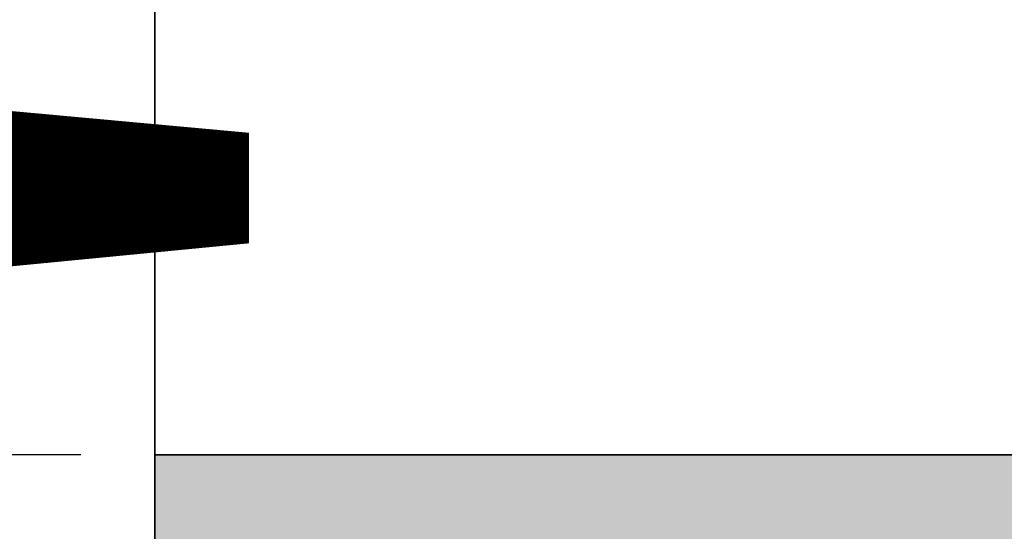
# Model space of a CAD drawing. Units: inches. Extents: x 2083 to 3317, y 1141 to 2115.
# Tile 22 of 256: x 2225.819 to 2234.135, y 1477.116 to 1481.434. Entities that reach past the tile are written whole.
import ezdxf

# ---------------------------------------------------------------- set-up
doc = ezdxf.new("R2010")
doc.units = ezdxf.units.IN
doc.layers.add('A-ANNO-DIMS', color=2, linetype='Continuous', lineweight=18)
doc.layers.add('A-WALL', color=7, linetype='Continuous', lineweight=35)
doc.layers.add('A-WALL-PATT', color=251, linetype='Continuous', lineweight=13, true_color=0x636466)
doc.styles.get("Standard").update_dxf_attribs({"font": 'arial.ttf'})
doc.dimstyles.new('ISO-25', dxfattribs={"dimtxt": 12, "dimasz": 12, "dimexe": 1.25, "dimexo": 0.625, "dimtad": 1, "dimlunit": 3, "dimtxsty": 'Standard', "dimcen": 2.5, "dimadec": 0, "dimazin": 0, "dimtfac": 1, "dimtmove": 0, "dimatfit": 3, "dimfxl": 1, "dimarcsym": 0})

# ---------------------------------------------------------------- blocks, each defined once
blk = doc.blocks.new('*D13')
at = {"layer": 'A-ANNO-DIMS', "color": 0, "lineweight": -2, "transparency": 16777216}
for p, q in [((2226.3348, 1477.7614), (2191.9761, 1477.7614)), ((2193.2261, 1465.7614), (2193.2261, 1275.2614)), ((2226.3348, 1263.2614), (2191.9761, 1263.2614))]:
    blk.add_line(p, q, dxfattribs=at)
at = {"layer": 'A-ANNO-DIMS', "color": 0, "transparency": 16777216}
for points in [[(2191.2261, 1465.7614), (2195.2261, 1465.7614), (2193.2261, 1477.7614)], [(2191.2261, 1275.2614), (2195.2261, 1275.2614), (2193.2261, 1263.2614)]]:
    blk.add_solid(points, dxfattribs=at)
at = {"layer": 'Defpoints', "color": 0, "transparency": 16777216}
for p in [(2226.9598, 1477.7614), (2193.2261, 1263.2614), (2226.9598, 1263.2614)]:
    blk.add_point(p, dxfattribs=at)
at = {"layer": 'A-ANNO-DIMS', "color": 0, "transparency": 16777216, "insert": (2186.4742, 1370.5114), "char_height": 12, "attachment_point": 5, "rotation": 90}
blk.add_mtext('17\'-10.5"', dxfattribs=at)
blk = doc.blocks.new('*D30')
at = {"layer": 'A-ANNO-DIMS', "color": 0, "lineweight": -2, "transparency": 16777216}
for p, q in [((2240.0179, 1445.2738), (2240.0179, 1448.0455)), ((2254.3293, 1445.2738), (2254.3293, 1448.0455)), ((2228.0179, 1446.7955), (2216.0179, 1446.7955)), ((2240.0179, 1446.7955), (2254.3293, 1446.7955)), ((2266.3293, 1446.7955), (2413.7649, 1446.7955))]:
    blk.add_line(p, q, dxfattribs=at)
at = {"layer": 'A-ANNO-DIMS', "color": 0, "transparency": 16777216}
for points in [[(2228.0179, 1448.7955), (2228.0179, 1444.7955), (2240.0179, 1446.7955)], [(2266.3293, 1448.7955), (2266.3293, 1444.7955), (2254.3293, 1446.7955)]]:
    blk.add_solid(points, dxfattribs=at)
at = {"layer": 'Defpoints', "color": 0, "transparency": 16777216}
for p in [(2254.3293, 1446.7955), (2240.0179, 1444.6488), (2254.3293, 1444.6488)]:
    blk.add_point(p, dxfattribs=at)
at = {"layer": 'A-ANNO-DIMS', "color": 0, "transparency": 16777216, "insert": (2346.0471, 1453.6252), "char_height": 12, "attachment_point": 5}
blk.add_mtext('WC 1\'-2 1/2" TYP.', dxfattribs=at)
blk = doc.blocks.new('*D31')
at = {"layer": 'A-ANNO-DIMS', "color": 0, "lineweight": -2, "transparency": 16777216}
for p, q in [((2237.8711, 1456.6488), (2237.8711, 1541.9152)), ((2239.3929, 1444.6488), (2236.6211, 1444.6488)), ((2237.8711, 1431.5475), (2237.8711, 1444.6488)), ((2239.3929, 1431.5475), (2236.6211, 1431.5475)), ((2237.8711, 1419.5475), (2237.8711, 1407.5475))]:
    blk.add_line(p, q, dxfattribs=at)
at = {"layer": 'A-ANNO-DIMS', "color": 0, "transparency": 16777216}
for points in [[(2235.8711, 1456.6488), (2239.8711, 1456.6488), (2237.8711, 1444.6488)], [(2235.8711, 1419.5475), (2239.8711, 1419.5475), (2237.8711, 1431.5475)]]:
    blk.add_solid(points, dxfattribs=at)
at = {"layer": 'Defpoints', "color": 0, "transparency": 16777216}
for p in [(2237.8711, 1444.6488), (2240.0179, 1444.6488), (2240.0179, 1431.5475)]:
    blk.add_point(p, dxfattribs=at)
at = {"layer": 'A-ANNO-DIMS', "color": 0, "transparency": 16777216, "insert": (2231.2175, 1505.282), "char_height": 12, "attachment_point": 5, "rotation": 90}
blk.add_mtext('1\'-1" TYP.', dxfattribs=at)

msp = doc.modelspace()

# ---------------------------------------------------------------- hatches: boundary and pattern name
at = {"layer": 'A-WALL-PATT'}
h = msp.add_hatch(color=256, dxfattribs=at)
h.dxf.hatch_style = 1
h.paths.add_polyline_path([(3126.9598, 2020.7614), (2748.9598, 2020.7614), (2604.9598, 2020.7614), (2226.9598, 2020.7614), (2226.9598, 1702.7614), (2466.9598, 1702.7614), (2466.9598, 1582.7614), (2418.9598, 1582.7614), (2418.9598, 1477.7614), (2226.9598, 1477.7614), (2226.9598, 1263.2614), (2544.9598, 1263.2614), (2544.9598, 1411.7614), (2604.9598, 1411.7614), (2685.9598, 1411.7614), (2685.9598, 1420.7614), (2604.9598, 1420.7614), (2604.9598, 1573.7614), (2604.9598, 1702.7614), (2604.9598, 2011.7614), (2748.9598, 2011.7614), (2748.9598, 1702.7614), (2862.9598, 1702.7614), (2862.9598, 1621.7614), (2871.9598, 1621.7614), (2871.9598, 1702.7614), (2883.9598, 1702.7614), (2883.9598, 1706.9395, -0.026459), (2883.9598, 1711.7614), (2757.9598, 1711.7614), (2757.9598, 1807.7614), (2787.9598, 1807.7614), (2787.9598, 1812.2614), (2757.9598, 1812.2614), (2757.9598, 2011.7614), (2877.9598, 2011.7614), (2877.9598, 1812.2614), (2847.9598, 1812.2614), (2847.9598, 1807.7614), (2889.8357, 1807.7614), (2889.8357, 1812.2614), (2882.4598, 1812.2614), (2882.4598, 2011.7614), (3117.9598, 2011.7614), (3117.9598, 1812.2614), (2937.8357, 1812.2614), (2937.8357, 1807.7614), (2995.7098, 1807.7614), (2995.7098, 1796.1177), (3000.2098, 1796.1177), (3000.2098, 1807.7614), (3117.9598, 1807.7614), (3117.9598, 1711.7614), (3000.2098, 1711.7614), (3000.2098, 1760.1177), (2998.5727, 1760.1177, -0.020711), (2995.7098, 1760.1177), (2995.7098, 1711.7614), (2931.9598, 1711.7614), (2931.9598, 1702.7614), (3126.9598, 1702.7614)])
h.paths.add_polyline_path([(2471.4598, 2011.7614), (2471.4598, 1810.0114), (2462.7169, 1810.0114), (2462.7169, 1805.5114), (2505.9598, 1805.5114), (2505.9598, 1810.0114), (2475.9598, 1810.0114), (2475.9598, 2011.7614), (2595.9598, 2011.7614), (2595.9598, 1810.0114), (2565.9598, 1810.0114), (2565.9598, 1805.5114), (2595.9598, 1805.5114), (2595.9598, 1711.7614), (2235.9598, 1711.7614), (2235.9598, 1805.5114), (2353.7098, 1805.5114), (2353.7098, 1796.0542), (2358.2098, 1796.0542), (2358.2098, 1805.5114), (2414.7169, 1805.5114), (2414.7169, 1810.0114), (2235.9598, 1810.0114), (2235.9598, 2011.7614)], flags=16)
h.paths.add_polyline_path([(2270.2047, 1994.61), (2270.2047, 1970.61), (2246.2047, 1970.61), (2246.2047, 1994.61)], flags=0)
edge = h.paths.add_edge_path(flags=0)
edge.add_ellipse((2332.0274, 1899.7982), major_axis=(-3.043, 3.043), ratio=0.168252, start_angle=-161.33217, end_angle=-156.30711, ccw=False)
edge.add_ellipse((2333.082, 1898.7435), major_axis=(-1.0546, 1.0546), ratio=0.453532, start_angle=-123.37102, end_angle=-94.15911)
edge = h.paths.add_edge_path(flags=0)
edge.add_ellipse((2332.0274, 1968.8763), major_axis=(3.043, 3.043), ratio=0.168252, start_angle=18.66783, end_angle=23.69289)
edge.add_spline(control_points=[(2332.9256, 1970.6911), (2332.2268, 1970.3361), (2330.8937, 1969.6589), (2328.4131, 1970.9321), (2327.2039, 1967.7487), (2324.7096, 1969.9556), (2322.5328, 1967.0124), (2320.0128, 1971.2958), (2317.6803, 1968.1578), (2316.0405, 1967.102), (2315.4269, 1966.8096)], knot_values=[0, 0, 0, 0, 2.267059, 4.324559, 6.685584, 8.878641, 11.121502, 14.300359, 17.755284, 19.732645, 19.732645, 19.732645, 19.732645], degree=3, periodic=0)
edge.add_ellipse((2332.0274, 1968.8763), major_axis=(3.043, 3.043), ratio=0.168252, start_angle=18.66783, end_angle=23.69289, ccw=False)
edge.add_ellipse((2333.082, 1969.9309), major_axis=(1.0546, 1.0546), ratio=0.453532, start_angle=56.62898, end_angle=85.84089, ccw=False)
edge = h.paths.add_edge_path(flags=0)
edge.add_spline(control_points=[(2296.4283, 1967.9879), (2293.6278, 1965.3363), (2287.7036, 1959.7271), (2299.7439, 1949.9957), (2294.5326, 1935.6685), (2290.5732, 1920.6035), (2293.3941, 1909.9737), (2296.1854, 1904.9665)], knot_values=[0.099185, 0.099185, 0.099185, 0.099185, 0.345301, 0.619822, 0.982653, 1.386093, 1.810555, 1.810555, 1.810555, 1.810555], degree=3, periodic=0)
edge.add_spline(control_points=[(2296.1854, 1904.9665), (2297.3836, 1902.6193), (2298.001, 1901.9493), (2298.553, 1901.4682)], knot_values=[0.006246, 0.006246, 0.006246, 0.006246, 0.055476, 0.055476, 0.055476, 0.055476], degree=3, periodic=0)
edge.add_spline(control_points=[(2298.553, 1901.4682), (2297.2586, 1900.9232), (2295.2253, 1900.2321), (2293.0602, 1900.6142), (2292.1014, 1900.7884), (2292.0896, 1900.7906)], knot_values=[0.312835, 0.312835, 0.312835, 0.312835, 0.40178, 0.474987, 0.475903, 0.475903, 0.475903, 0.475903], degree=3, periodic=0)
edge.add_arc((2292.7936, 1904.6641), 3.937, 215.4209, 259.69818, ccw=False)
edge.add_spline(control_points=[(2289.5853, 1902.3823), (2289.4767, 1902.5351), (2289.3685, 1902.688), (2289.2609, 1902.8412)], knot_values=[0.102872, 0.102872, 0.102872, 0.102872, 0.116896, 0.116896, 0.116896, 0.116896], degree=3, periodic=0)
edge.add_spline(control_points=[(2289.2609, 1902.8412), (2288.6866, 1902.5502), (2287.64, 1902.0199), (2285.8813, 1901.874), (2283.853, 1901.5044), (2281.72, 1899.7105), (2278.467, 1899.4929), (2276.1571, 1901.8832), (2272.259, 1899.8041), (2267.7776, 1901.8432), (2262.2439, 1900.184), (2257.4149, 1901.7821), (2254.3184, 1900.7261), (2253.1783, 1900.3373)], knot_values=[0, 0, 0, 0, 1.907977, 3.477176, 5.261074, 7.972851, 11.680248, 13.717921, 16.939592, 22.789562, 27.502503, 33.595215, 37.145618, 37.145618, 37.145618, 37.145618], degree=3, periodic=0)
edge.add_line((2253.1783, 1900.3373), (2250.2442, 1902.8412))
edge.add_line((2250.2442, 1902.8412), (2250.2442, 1965.8333))
edge.add_line((2250.2442, 1965.8333), (2253.1783, 1968.3371))
edge.add_spline(control_points=[(2253.1783, 1968.3371), (2254.3184, 1967.9483), (2257.4149, 1966.8924), (2262.2439, 1968.4904), (2267.7776, 1966.8313), (2271.5267, 1968.5372), (2273.8759, 1967.8283), (2274.2067, 1967.7276)], knot_values=[0, 0, 0, 0, 0.09018, 0.244935, 0.364644, 0.513233, 0.537855, 0.537855, 0.537855, 0.537855], degree=3, periodic=0)
edge.add_arc((2274.3529, 1963.7933), 3.937, 72.05113, 92.12795, ccw=False)
edge.add_arc((2281.2969, 1985.23), 18.5963, 252.05113, 288.56572)
edge.add_arc((2292.3167, 1956.0289), 12.6461, 71.02679, 113.77822, ccw=False)
edge = h.paths.add_edge_path(flags=0)
edge.add_spline(control_points=[(2274.8994, 1951.8562), (2275.0662, 1951.6166), (2275.2327, 1951.3766), (2275.398, 1951.1359)], knot_values=[1.409916, 1.409916, 1.409916, 1.409916, 1.43159, 1.43159, 1.43159, 1.43159], degree=3, periodic=0)
edge.add_spline(control_points=[(2275.398, 1951.1359), (2275.7921, 1950.5619), (2276.1792, 1949.9838), (2276.5455, 1949.3971)], knot_values=[1.358238, 1.358238, 1.358238, 1.358238, 1.409916, 1.409916, 1.409916, 1.409916], degree=3, periodic=0)
edge.add_line((2276.5455, 1949.3971), (2277.4373, 1947.8622))
edge.add_spline(control_points=[(2277.4373, 1947.8622), (2276.3038, 1945.6731), (2274.6397, 1942.4269), (2274.6316, 1938.0939), (2272.7991, 1930.8515), (2274.3564, 1943.897), (2275.9477, 1947.9234), (2276.5455, 1949.3971)], knot_values=[0.005632, 0.005632, 0.005632, 0.005632, 0.186014, 0.266002, 0.357087, 0.59639, 0.739732, 0.739732, 0.739732, 0.739732], degree=3, periodic=0)
edge.add_spline(control_points=[(2276.5455, 1949.3971), (2276.1792, 1949.9838), (2275.7921, 1950.5619), (2275.398, 1951.1359)], knot_values=[1.358238, 1.358238, 1.358238, 1.358238, 1.409916, 1.409916, 1.409916, 1.409916], degree=3, periodic=0)
edge.add_spline(control_points=[(2275.398, 1951.1359), (2274.9425, 1950.0805), (2274.2078, 1948.0253), (2273.9346, 1944.8515), (2272.4685, 1937.6275), (2273.4662, 1945.6965), (2274.7006, 1951.0595), (2274.8994, 1951.8562)], knot_values=[0.104364, 0.104364, 0.104364, 0.104364, 0.189636, 0.269624, 0.36071, 0.600013, 0.644622, 0.644622, 0.644622, 0.644622], degree=3, periodic=0)
h.paths.add_polyline_path([(2269.1675, 1963.1276, -0.357527), (2268.1706, 1960.9764, -0.092561), (2268.1706, 1939.4363, -0.357527), (2269.1675, 1937.2851, -0.357527), (2267.0163, 1938.282, -0.164785), (2254.6856, 1938.282, -0.357527), (2252.5344, 1937.2851, -0.357527), (2253.5313, 1939.4363, -0.092561), (2253.5313, 1960.9764, -0.357527), (2252.5344, 1963.1276, -0.357527), (2254.6856, 1962.1307, -0.164785), (2267.0163, 1962.1307, -0.357527)], flags=0)
h.paths.add_polyline_path([(2248.8741, 1967.8018), (2248.8741, 1957.0277), (2249.4578, 1957.0277), (2249.4578, 1911.6468), (2248.8741, 1911.6468), (2248.8741, 1900.8727), (2246.5119, 1900.8727, 0.197327), (2244.1497, 1902.4569), (2244.1497, 1966.2176, 0.197327), (2246.5119, 1967.8018)], flags=0)
h.paths.add_polyline_path([(2269.1675, 1931.3893, -0.357527), (2268.1706, 1929.2381, -0.092561), (2268.1706, 1907.6981, -0.357527), (2269.1675, 1905.5469, -0.357527), (2267.0163, 1906.5438, -0.164785), (2254.6856, 1906.5438, -0.357527), (2252.5344, 1905.5469, -0.357527), (2253.5313, 1907.6981, -0.092561), (2253.5313, 1929.2381, -0.357527), (2252.5344, 1931.3893, -0.357527), (2254.6856, 1930.3925, -0.164785), (2267.0163, 1930.3925, -0.357527)], flags=0)
edge = h.paths.add_edge_path(flags=0)
edge.add_spline(control_points=[(2276.1969, 1906.7237), (2276.1681, 1909.0289), (2276.114, 1913.3719), (2270.5984, 1924.925), (2273.9052, 1919.0128), (2275.9217, 1916.2621), (2275.4746, 1912.4021), (2277.2579, 1910.3806), (2276.696, 1908.225), (2276.6462, 1906.813), (2276.6178, 1906.0084)], knot_values=[0, 0, 0, 0, 8.61026, 16.221274, 18.843057, 23.804898, 27.440828, 29.356102, 31.203478, 33.650687, 33.650687, 33.650687, 33.650687], degree=3, periodic=0)
edge.add_spline(control_points=[(2276.6178, 1906.0084), (2276.6233, 1905.6241), (2276.4977, 1904.6287), (2275.4418, 1903.8547), (2274.9373, 1903.0804), (2274.8591, 1902.8412)], knot_values=[0.156488, 0.156488, 0.156488, 0.156488, 0.184398, 0.231376, 0.250598, 0.250598, 0.250598, 0.250598], degree=3, periodic=0)
edge.add_line((2274.8591, 1902.8412), (2276.506, 1902.8412))
edge.add_spline(control_points=[(2276.506, 1902.8412), (2276.7883, 1903.0849), (2277.6651, 1904.1252), (2278.2495, 1904.3407), (2277.6539, 1908.5274), (2278.1557, 1906.2278), (2278.1005, 1905.2859), (2278.8467, 1904.069), (2277.8568, 1903.4149), (2277.8742, 1902.991), (2277.9036, 1902.8412)], knot_values=[0.059574, 0.059574, 0.059574, 0.059574, 0.080753, 0.103741, 0.16972, 0.176036, 0.207137, 0.240474, 0.262341, 0.27366, 0.27366, 0.27366, 0.27366], degree=3, periodic=0)
edge.add_line((2277.9036, 1902.8412), (2280.0298, 1902.8412))
edge.add_spline(control_points=[(2280.0298, 1902.8412), (2279.8882, 1903.0884), (2279.4993, 1903.9816), (2280.1523, 1905.9393), (2278.1036, 1909.6578), (2279.7624, 1907.1853), (2280.3279, 1904.8749), (2280.4851, 1903.4896), (2281.4633, 1903.2494), (2281.7583, 1902.9365), (2281.834, 1902.8412)], knot_values=[0.013856, 0.013856, 0.013856, 0.013856, 0.034874, 0.088867, 0.107879, 0.126738, 0.158714, 0.193757, 0.217487, 0.226722, 0.226722, 0.226722, 0.226722], degree=3, periodic=0)
edge.add_spline(control_points=[(2281.834, 1902.8412), (2281.7875, 1902.8267), (2281.647, 1902.783), (2281.3955, 1902.8595), (2281.0881, 1902.9852), (2280.7207, 1903.0609), (2280.3335, 1903.0257), (2280.1248, 1902.8989), (2280.0298, 1902.8412)], knot_values=[0, 0, 0, 0, 0.14413, 0.435517, 0.749276, 1.153046, 1.548371, 1.878348, 1.878348, 1.878348, 1.878348], degree=3, periodic=0)
edge.add_line((2280.0298, 1902.8412), (2277.9036, 1902.8412))
edge.add_spline(control_points=[(2277.9036, 1902.8412), (2277.8929, 1902.7959), (2277.8654, 1902.6796), (2277.6075, 1902.6875), (2277.2741, 1902.8007), (2276.8379, 1902.6198), (2276.5838, 1902.7893), (2276.506, 1902.8412)], knot_values=[0, 0, 0, 0, 0.127189, 0.326199, 0.628009, 1.24357, 1.515331, 1.515331, 1.515331, 1.515331], degree=3, periodic=0)
edge.add_line((2276.506, 1902.8412), (2274.8591, 1902.8412))
edge.add_spline(control_points=[(2274.8591, 1902.8412), (2274.8144, 1902.8986), (2274.7251, 1903.0134), (2274.4935, 1903.119), (2274.2443, 1902.9605), (2273.9371, 1903.1849), (2273.614, 1902.9831), (2273.4083, 1902.883), (2273.3223, 1902.8412)], knot_values=[0, 0, 0, 0, 0.21843, 0.436957, 0.687977, 0.990379, 1.398396, 1.69185, 1.69185, 1.69185, 1.69185], degree=3, periodic=0)
edge.add_spline(control_points=[(2273.3223, 1902.8412), (2273.6167, 1903.4457), (2274.274, 1904.5383), (2276.0272, 1904.5737), (2276.207, 1906.5836), (2276.1969, 1906.7237)], knot_values=[0.012227, 0.012227, 0.012227, 0.012227, 0.059472, 0.106218, 0.134458, 0.134458, 0.134458, 0.134458], degree=3, periodic=0)
h.paths.add_polyline_path([(2270.7761, 1897.7898), (2270.7761, 1873.7898), (2246.7761, 1873.7898), (2246.7761, 1897.7898)], flags=0)
h.paths.add_polyline_path([(2353.7098, 1760.0051), (2353.7098, 1760.0542), (2358.2098, 1760.0542, -0.033729)], flags=0)
h.paths.add_polyline_path([(2321.8191, 1737.5292), (2341.9953, 1737.5292, -0.414214), (2343.2033, 1736.3212), (2343.2033, 1721.0206, -0.414214), (2341.9953, 1719.8127), (2321.8191, 1719.8127, -0.414214), (2320.6112, 1721.0206), (2320.6112, 1736.3212, -0.414214)], flags=0)
h.paths.add_polyline_path([(2324.235, 1736.3212), (2339.5794, 1736.3212, -0.414214), (2341.9953, 1733.9053), (2341.9953, 1725.4497, -0.414214), (2339.5794, 1723.0338), (2333.6806, 1723.0338), (2333.8453, 1722.0455, -0.870646), (2335.4254, 1721.8259, -0.767327), (2333.9227, 1721.4232), (2331.291, 1721.4232, -0.767327), (2329.7883, 1721.8259, -0.870646), (2331.3684, 1722.0455), (2331.5331, 1723.0338), (2324.235, 1723.0338, -0.414214), (2321.8191, 1725.4497), (2321.8191, 1733.9053, -0.414214)], flags=0)
h.paths.add_polyline_path([(2570.4838, 1928.6154), (2589.6838, 1928.6154), (2590.1688, 1928.6154), (2590.1688, 1904.9934), (2570.4838, 1904.9934)], flags=0)
h.paths.add_polyline_path([(2574.4473, 1927.2638, -1), (2572.8288, 1927.2638, -1)], flags=0)
h.paths.add_polyline_path([(2573.0899, 1926.9409), (2573.925, 1927.776), (2574.1477, 1927.5533), (2573.3126, 1926.7182)], flags=0)
h.paths.add_polyline_path([(2578.7791, 1919.7296, -1), (2571.5917, 1919.7296, -1)], flags=0)
h.paths.add_polyline_path([(2578.3854, 1919.7296, -1), (2571.9854, 1919.7296, -1)], flags=0)
h.paths.add_polyline_path([(2331.5958, 1729.4762, -1), (2333.618, 1729.4762, -1)], flags=0)
h.paths.add_polyline_path([(2578.0342, 1927.2638, -1), (2576.4157, 1927.2638, -1)], flags=0)
h.paths.add_polyline_path([(2576.6889, 1927.5311), (2576.9116, 1927.7538), (2577.7467, 1926.9186), (2577.524, 1926.6959)], flags=0)
h.paths.add_polyline_path([(2578.1391, 1909.8595, -1), (2572.2317, 1909.8595, -1)], flags=0)
h.paths.add_polyline_path([(2577.7454, 1909.8595, -1), (2572.6254, 1909.8595, -1)], flags=0)
h.paths.add_polyline_path([(2583.7977, 1927.2638, -1), (2582.1792, 1927.2638, -1)], flags=0)
h.paths.add_polyline_path([(2582.7186, 1927.7538), (2583.5538, 1926.9186), (2583.3311, 1926.6959), (2582.4959, 1927.5311)], flags=0)
h.paths.add_polyline_path([(2582.4959, 1927.5311), (2582.7186, 1927.7538), (2583.5538, 1926.9186), (2583.3311, 1926.6959)], flags=0)
h.paths.add_polyline_path([(2587.7391, 1920.5296, -1), (2581.8317, 1920.5296, -1)], flags=0)
h.paths.add_polyline_path([(2587.3454, 1920.5296, -1), (2582.2254, 1920.5296, -1)], flags=0)
h.paths.add_polyline_path([(2587.3846, 1927.2638, -1), (2585.7661, 1927.2638, -1)], flags=0)
h.paths.add_polyline_path([(2586.082, 1926.9802), (2586.9172, 1927.8154), (2587.1399, 1927.5927), (2586.3047, 1926.7575)], flags=0)
h.paths.add_polyline_path([(2588.3791, 1910.6595, -1), (2581.1917, 1910.6595, -1)], flags=0)
h.paths.add_polyline_path([(2587.9854, 1910.6595, -1), (2581.5854, 1910.6595, -1)], flags=0)
h.paths.add_polyline_path([(2417.1677, 1729.4779), (2437.3439, 1729.4779, -0.414214), (2438.5519, 1728.2699), (2438.5519, 1712.9693, -0.414214), (2437.3439, 1711.7614), (2417.1677, 1711.7614, -0.414214), (2415.9598, 1712.9693), (2415.9598, 1728.2699, -0.414214)], flags=0)
h.paths.add_polyline_path([(2419.5836, 1728.2699), (2434.928, 1728.2699, -0.414214), (2437.3439, 1725.8541), (2437.3439, 1717.3984, -0.414214), (2434.928, 1714.9825), (2429.0292, 1714.9825), (2429.1939, 1713.9942, -0.870646), (2430.774, 1713.7746, -0.767327), (2429.2713, 1713.372), (2426.6396, 1713.372, -0.767327), (2425.1369, 1713.7746, -0.870646), (2426.717, 1713.9942), (2426.8817, 1714.9825), (2419.5836, 1714.9825, -0.414214), (2417.1677, 1717.3984), (2417.1677, 1725.8541, -0.414214)], flags=0)
h.paths.add_polyline_path([(2419.5836, 1728.2699), (2434.928, 1728.2699, -0.414214), (2437.3439, 1725.8541), (2437.3439, 1717.3984, -0.414214), (2434.928, 1714.9825), (2429.0292, 1714.9825), (2428.3581, 1719.009), (2427.5528, 1719.009), (2426.8817, 1714.9825), (2419.5836, 1714.9825, -0.414214), (2417.1677, 1717.3984), (2417.1677, 1725.8541, -0.414214)], flags=0)
h.paths.add_polyline_path([(2426.9444, 1721.4249, -1), (2428.9666, 1721.4249, -1)], flags=0)
h.paths.add_polyline_path([(2475.9598, 1702.7614), (2595.9598, 1702.7614), (2595.9598, 1582.7614), (2475.9598, 1582.7614)], flags=16)
h.paths.add_polyline_path([(2427.9598, 1573.7614), (2595.9598, 1573.7614), (2595.9598, 1468.7614), (2595.9598, 1420.7614), (2384.4598, 1420.7614), (2384.4598, 1468.7614), (2427.9598, 1468.7614)], flags=16)
h.paths.add_polyline_path([(2379.9598, 1468.7614), (2379.9598, 1420.7614), (2235.9598, 1420.7614), (2235.9598, 1468.7614)], flags=16)
h.paths.add_polyline_path([(2317.816, 1466.6958), (2337.9922, 1466.6958, -0.414214), (2339.2002, 1465.4878), (2339.2002, 1450.1872, -0.414214), (2337.9922, 1448.9792), (2317.816, 1448.9792, -0.414214), (2316.6081, 1450.1872), (2316.6081, 1465.4878, -0.414214)], flags=0)
h.paths.add_polyline_path([(2320.2319, 1465.4878), (2335.5763, 1465.4878, -0.414214), (2337.9922, 1463.0719), (2337.9922, 1454.6163, -0.414214), (2335.5763, 1452.2004), (2329.6775, 1452.2004), (2329.8422, 1451.212, -0.870646), (2331.4223, 1450.9925, -0.767327), (2329.9196, 1450.5898), (2327.2879, 1450.5898, -0.767327), (2325.7852, 1450.9925, -0.870646), (2327.3653, 1451.212), (2327.53, 1452.2004), (2320.2319, 1452.2004, -0.414214), (2317.816, 1454.6163), (2317.816, 1463.0719, -0.414214)], flags=0)
h.paths.add_polyline_path([(2320.2319, 1465.4878), (2335.5763, 1465.4878, -0.414214), (2337.9922, 1463.0719), (2337.9922, 1454.6163, -0.414214), (2335.5763, 1452.2004), (2329.6775, 1452.2004), (2329.0064, 1456.2269), (2328.2011, 1456.2269), (2327.53, 1452.2004), (2320.2319, 1452.2004, -0.414214), (2317.816, 1454.6163), (2317.816, 1463.0719, -0.414214)], flags=0)
h.paths.add_polyline_path([(2327.5926, 1458.6428, -1), (2329.6148, 1458.6428, -1)], flags=0)
h.paths.add_polyline_path([(2244.4117, 1433.3405), (2241.9209, 1433.3405, -0.414214), (2240.0179, 1435.2435), (2240.0179, 1440.9528, -0.414211), (2241.9209, 1442.8559), (2244.4117, 1442.8559, -1.976472)], flags=0)
h.paths.add_polyline_path([(2245.3569, 1434.3975, -0.414214), (2245.3569, 1441.7988, -2.144098)], flags=0)
h.paths.add_polyline_path([(2535.9598, 1416.2614), (2535.9598, 1272.2614), (2235.9598, 1272.2614), (2235.9598, 1416.2614)], flags=16)
h.paths.add_polyline_path([(2260.1196, 1384.2928), (2260.1196, 1362.0386), (2237.8654, 1362.0386), (2237.8654, 1384.2928)], flags=0)
edge = h.paths.add_edge_path(flags=0)
edge.add_line((2318.2518, 1362.0933), (2318.1458, 1362.001))
edge.add_ellipse((2317.4451, 1360.431), major_axis=(2.8216, 2.8216), ratio=0.168252, start_angle=18.66783, end_angle=20.94813, ccw=False)
edge.add_ellipse((2318.423, 1361.409), major_axis=(0.9779, 0.9779), ratio=0.453532, start_angle=56.62898, end_angle=70.2262, ccw=False)
edge = h.paths.add_edge_path(flags=0)
edge.add_line((2319.1074, 1295.5711), (2319.015, 1295.6771))
edge.add_ellipse((2317.4451, 1296.3778), major_axis=(-2.8216, 2.8216), ratio=0.168252, start_angle=-161.33217, end_angle=-159.05187, ccw=False)
edge.add_ellipse((2318.423, 1295.3999), major_axis=(-0.9779, 0.9779), ratio=0.453532, start_angle=-123.37102, end_angle=-109.7738)
edge = h.paths.add_edge_path(flags=0)
edge.add_spline(control_points=[(2284.2103, 1301.1702), (2284.5807, 1300.4447), (2284.8912, 1299.892), (2285.1596, 1299.461)], knot_values=[0.039066, 0.039066, 0.039066, 0.039066, 0.055476, 0.055476, 0.055476, 0.055476], degree=3, periodic=0)
edge.add_line((2285.1596, 1299.461), (2284.2103, 1301.1702))
edge = h.paths.add_edge_path(flags=0)
edge.add_line((2280.4125, 1297.298), (2283.37, 1297.0361))
edge.add_line((2283.37, 1297.0361), (2286.4057, 1297.9263))
edge.add_spline(control_points=[(2286.4057, 1297.9263), (2285.3055, 1297.4631), (2284.3448, 1297.1292), (2283.37, 1297.0361)], knot_values=[0.394369, 0.394369, 0.394369, 0.394369, 0.475903, 0.475903, 0.475903, 0.475903], degree=3, periodic=0)
edge.add_spline(control_points=[(2283.37, 1297.0361), (2283.2814, 1297.0277), (2282.3163, 1296.9573), (2281.3125, 1297.1345), (2280.4234, 1297.296), (2280.4125, 1297.298)], knot_values=[0.312835, 0.312835, 0.312835, 0.312835, 0.320246, 0.393453, 0.394369, 0.394369, 0.394369, 0.394369], degree=3, periodic=0)
edge = h.paths.add_edge_path(flags=0)
edge.add_line((2284.4356, 1359.6073), (2280.4463, 1355.328))
edge.add_line((2280.4463, 1355.328), (2279.58, 1351.0178))
edge.add_line((2279.58, 1351.0178), (2282.413, 1346.5804))
edge.add_spline(control_points=[(2282.413, 1346.5804), (2283.1533, 1345.5892), (2284.2529, 1344.0289), (2284.801, 1342.3872), (2284.9352, 1341.8055)], knot_values=[1.240098, 1.240098, 1.240098, 1.240098, 1.332892, 1.382712, 1.382712, 1.382712, 1.382712], degree=3, periodic=0)
edge.add_spline(control_points=[(2284.9352, 1341.8055), (2285.3191, 1340.1406), (2285.233, 1338.4092), (2284.9099, 1336.6541)], knot_values=[1.097484, 1.097484, 1.097484, 1.097484, 1.240098, 1.240098, 1.240098, 1.240098], degree=3, periodic=0)
edge.add_spline(control_points=[(2284.9099, 1336.6541), (2284.5868, 1334.899), (2284.0267, 1333.1203), (2283.4626, 1331.3606)], knot_values=[0.95487, 0.95487, 0.95487, 0.95487, 1.097484, 1.097484, 1.097484, 1.097484], degree=3, periodic=0)
edge.add_line((2283.4626, 1331.3606), (2281.8904, 1326.1534))
edge.add_line((2281.8904, 1326.1534), (2280.7563, 1321.0561))
edge.add_line((2280.7563, 1321.0561), (2280.2992, 1316.002))
edge.add_line((2280.2992, 1316.002), (2280.7159, 1310.9501))
edge.add_line((2280.7159, 1310.9501), (2282.0281, 1305.9721))
edge.add_line((2282.0281, 1305.9721), (2284.2103, 1301.1702))
edge.add_spline(control_points=[(2284.2103, 1301.1702), (2283.3407, 1302.7302), (2282.6119, 1304.3365), (2282.0281, 1305.9721)], knot_values=[0.099185, 0.099185, 0.099185, 0.099185, 0.241799, 0.241799, 0.241799, 0.241799], degree=3, periodic=0)
edge.add_spline(control_points=[(2282.0281, 1305.9721), (2281.4443, 1307.6078), (2281.0055, 1309.2728), (2280.7159, 1310.9501)], knot_values=[0.241799, 0.241799, 0.241799, 0.241799, 0.384413, 0.384413, 0.384413, 0.384413], degree=3, periodic=0)
edge.add_spline(control_points=[(2280.7159, 1310.9501), (2280.4332, 1312.5876), (2280.2894, 1314.277), (2280.2989, 1315.962), (2280.2992, 1316.002)], knot_values=[0.384413, 0.384413, 0.384413, 0.384413, 0.523647, 0.527028, 0.527028, 0.527028, 0.527028], degree=3, periodic=0)
edge.add_spline(control_points=[(2280.2992, 1316.002), (2280.3123, 1317.687), (2280.4779, 1319.3679), (2280.7563, 1321.0561)], knot_values=[0.527028, 0.527028, 0.527028, 0.527028, 0.669642, 0.669642, 0.669642, 0.669642], degree=3, periodic=0)
edge.add_spline(control_points=[(2280.7563, 1321.0561), (2281.0346, 1322.7443), (2281.4259, 1324.4396), (2281.8904, 1326.1534)], knot_values=[0.669642, 0.669642, 0.669642, 0.669642, 0.812256, 0.812256, 0.812256, 0.812256], degree=3, periodic=0)
edge.add_spline(control_points=[(2281.8904, 1326.1534), (2282.2644, 1327.5333), (2282.7879, 1329.2618), (2283.3528, 1331.0178), (2283.4626, 1331.3606)], knot_values=[0.812256, 0.812256, 0.812256, 0.812256, 0.927087, 0.95487, 0.95487, 0.95487, 0.95487], degree=3, periodic=0)
edge.add_line((2283.4626, 1331.3606), (2284.9099, 1336.6541))
edge.add_line((2284.9099, 1336.6541), (2284.9352, 1341.8055))
edge.add_line((2284.9352, 1341.8055), (2282.413, 1346.5804))
edge.add_spline(control_points=[(2282.413, 1346.5804), (2281.2751, 1348.1038), (2280.0784, 1349.5703), (2279.58, 1351.0178)], knot_values=[1.382712, 1.382712, 1.382712, 1.382712, 1.525326, 1.525326, 1.525326, 1.525326], degree=3, periodic=0)
edge.add_spline(control_points=[(2279.58, 1351.0178), (2279.4433, 1351.4147), (2279.1363, 1352.8569), (2279.7352, 1354.2904), (2280.4463, 1355.328)], knot_values=[1.525326, 1.525326, 1.525326, 1.525326, 1.564439, 1.667941, 1.667941, 1.667941, 1.667941], degree=3, periodic=0)
edge.add_spline(control_points=[(2280.4463, 1355.328), (2281.4261, 1356.7578), (2282.9308, 1358.1826), (2284.4356, 1359.6073)], knot_values=[1.667941, 1.667941, 1.667941, 1.667941, 1.810555, 1.810555, 1.810555, 1.810555], degree=3, periodic=0)
edge.add_arc((2280.6231, 1348.5182), 11.7262, 71.02679, 113.77822)
edge.add_arc((2270.4049, 1375.5952), 17.2436, 252.05113, 288.56572, ccw=False)
edge.add_arc((2263.966, 1355.7178), 3.6506, 72.05113, 92.12795)
edge.add_arc((2263.966, 1355.7178), 3.6506, 92.12795, 177.98513)
edge.add_spline(control_points=[(2260.3176, 1355.8462), (2260.2604, 1354.2207), (2260.5513, 1350.1865), (2262.9993, 1346.7663), (2264.4727, 1344.649)], knot_values=[1.43159, 1.43159, 1.43159, 1.43159, 1.564144, 1.770695, 1.770695, 1.770695, 1.770695], degree=3, periodic=0)
edge.add_line((2264.4727, 1344.649), (2264.9356, 1343.9825))
edge.add_spline(control_points=[(2263.801, 1340.2481), (2263.8432, 1340.5141), (2264.0672, 1341.7565), (2264.5127, 1343.0025), (2264.935, 1343.9811)], knot_values=[0.53657, 0.53657, 0.53657, 0.53657, 0.559349, 0.644622, 0.644622, 0.644622, 0.644622], degree=3, periodic=0)
edge.add_spline(control_points=[(2264.935, 1343.9811), (2265.1178, 1343.715), (2265.2989, 1343.4479), (2265.4768, 1343.1794)], knot_values=[1.384077, 1.384077, 1.384077, 1.384077, 1.409916, 1.409916, 1.409916, 1.409916], degree=3, periodic=0)
edge.add_spline(control_points=[(2265.4768, 1343.1794), (2265.6546, 1342.9108), (2265.8293, 1342.6408), (2265.9991, 1342.3688)], knot_values=[1.358238, 1.358238, 1.358238, 1.358238, 1.384077, 1.384077, 1.384077, 1.384077], degree=3, periodic=0)
edge.add_line((2265.9991, 1342.3688), (2266.826, 1340.9455))
edge.add_spline(control_points=[(2266.826, 1340.9455), (2268.8944, 1337.0897), (2271.3982, 1325.843), (2270.5162, 1310.5686), (2275.9194, 1301.8606), (2277.7895, 1299.1994)], knot_values=[0.116896, 0.116896, 0.116896, 0.116896, 0.472987, 1.050969, 1.313793, 1.313793, 1.313793, 1.313793], degree=3, periodic=0)
edge.add_spline(control_points=[(2277.7895, 1299.1994), (2277.8394, 1299.1285), (2277.8894, 1299.0575), (2277.9396, 1298.9866)], knot_values=[0.109884, 0.109884, 0.109884, 0.109884, 0.116896, 0.116896, 0.116896, 0.116896], degree=3, periodic=0)
edge.add_line((2277.9396, 1298.9866), (2277.7888, 1299.1991))
edge.add_spline(control_points=[(2277.7888, 1299.1991), (2277.2566, 1298.9294), (2276.2864, 1298.4379), (2275.0394, 1298.3344), (2274.3833, 1298.2389), (2274.2153, 1298.2093)], knot_values=[33.12187, 33.12187, 33.12187, 33.12187, 35.029056, 36.598255, 37.144827, 37.144827, 37.144827, 37.144827], degree=3, periodic=0)
edge.add_line((2274.2153, 1298.2093), (2273.0731, 1297.893))
edge.add_spline(control_points=[(2273.0731, 1297.893), (2272.3229, 1297.5798), (2271.0392, 1296.5105), (2269.2484, 1296.2261), (2268.4231, 1296.3747)], knot_values=[26.532584, 26.532584, 26.532584, 26.532584, 29.198919, 31.839101, 31.839101, 31.839101, 31.839101], degree=3, periodic=0)
edge.add_line((2268.4231, 1296.3747), (2263.8785, 1297.4575))
edge.add_spline(control_points=[(2263.8785, 1297.4575), (2263.5561, 1297.3594), (2261.8603, 1296.8387), (2260.2388, 1297.2824), (2258.9335, 1297.5165)], knot_values=[15.919551, 15.919551, 15.919551, 15.919551, 16.939592, 21.226067, 21.226067, 21.226067, 21.226067], degree=3, periodic=0)
edge.add_line((2258.9335, 1297.5165), (2254.0552, 1297.329))
edge.add_spline(control_points=[(2254.0552, 1297.329), (2253.7555, 1297.2958), (2252.1137, 1297.1652), (2250.4619, 1297.5442), (2249.1297, 1297.6679)], knot_values=[5.306517, 5.306517, 5.306517, 5.306517, 6.276435, 10.613034, 10.613034, 10.613034, 10.613034], degree=3, periodic=0)
edge.add_line((2249.1297, 1297.6679), (2244.3316, 1296.8778))
edge.add_line((2244.3316, 1296.8778), (2241.611, 1299.1994))
edge.add_line((2241.611, 1299.1994), (2241.611, 1357.6094))
edge.add_line((2241.611, 1357.6094), (2244.3316, 1359.9311))
edge.add_line((2244.3316, 1359.9311), (2252.7288, 1359.5427))
edge.add_spline(control_points=[(2252.7288, 1359.5427), (2252.8709, 1359.5464), (2253.3057, 1359.5482), (2253.7398, 1359.5143), (2254.0317, 1359.4824)], knot_values=[0.233291, 0.233291, 0.233291, 0.233291, 0.244935, 0.268927, 0.268927, 0.268927, 0.268927], degree=3, periodic=0)
edge.add_line((2254.0317, 1359.4824), (2259.5872, 1359.4164))
edge.add_spline(control_points=[(2259.5872, 1359.4164), (2260.6771, 1359.6285), (2262.0732, 1359.897), (2263.5237, 1359.4593), (2263.8304, 1359.366)], knot_values=[0.422516, 0.422516, 0.422516, 0.422516, 0.513233, 0.537855, 0.537855, 0.537855, 0.537855], degree=3, periodic=0)
edge.add_arc((2263.966, 1355.7178), 3.6506, 72.05113, 92.12795, ccw=False)
edge.add_arc((2270.4049, 1375.5952), 17.2436, 252.05113, 288.56572)
edge.add_arc((2280.6231, 1348.5182), 11.7262, 71.02679, 113.77822, ccw=False)
h.paths.add_polyline_path([(2240.3405, 1359.4347), (2240.3405, 1349.4444), (2240.8818, 1349.4444), (2240.8818, 1307.3645), (2240.3405, 1307.3645), (2240.3405, 1297.3741), (2238.1502, 1297.3741, 0.197327), (2235.9598, 1298.8431), (2235.9598, 1357.9657, 0.197327), (2238.1502, 1359.4347)], flags=0)
h.paths.add_polyline_path([(2259.1578, 1355.1005, -0.357527), (2258.2334, 1353.1058, -0.092561), (2258.2334, 1333.1326, -0.357527), (2259.1578, 1331.1379, -0.357527), (2257.1631, 1332.0622, -0.164785), (2245.7293, 1332.0622, -0.357527), (2243.7346, 1331.1379, -0.357527), (2244.6589, 1333.1326, -0.092561), (2244.6589, 1353.1058, -0.357527), (2243.7346, 1355.1005, -0.357527), (2245.7293, 1354.1761, -0.164785), (2257.1631, 1354.1761, -0.357527)], flags=0)
edge = h.paths.add_edge_path(flags=0)
edge.add_line((2265.9991, 1342.3688), (2266.826, 1340.9455))
edge.add_line((2266.826, 1340.9455), (2265.3076, 1337.8141))
edge.add_line((2265.3076, 1337.8141), (2264.3582, 1334.6529))
edge.add_line((2264.3582, 1334.6529), (2264.262, 1333.7997))
edge.add_spline(control_points=[(2264.262, 1333.7997), (2264.2084, 1333.1871), (2264.1621, 1332.3655), (2264.0071, 1331.4139), (2263.969, 1331.2018)], knot_values=[0.464444, 0.464444, 0.464444, 0.464444, 0.516691, 0.531608, 0.531608, 0.531608, 0.531608], degree=3, periodic=0)
edge.add_spline(control_points=[(2263.969, 1331.2018), (2263.7745, 1330.1189), (2263.4244, 1328.7908), (2263.2574, 1328.5307), (2263.234, 1328.5146)], knot_values=[0.372682, 0.372682, 0.372682, 0.372682, 0.44885, 0.464444, 0.464444, 0.464444, 0.464444], degree=3, periodic=0)
edge.add_spline(control_points=[(2263.234, 1328.5146), (2263.0964, 1328.4202), (2263.1312, 1329.3015), (2263.275, 1330.6157)], knot_values=[0.280919, 0.280919, 0.280919, 0.280919, 0.372682, 0.372682, 0.372682, 0.372682], degree=3, periodic=0)
edge.add_spline(control_points=[(2263.275, 1330.6157), (2263.4187, 1331.93), (2263.6715, 1333.6773), (2263.9699, 1335.315)], knot_values=[0.189157, 0.189157, 0.189157, 0.189157, 0.280919, 0.280919, 0.280919, 0.280919], degree=3, periodic=0)
edge.add_spline(control_points=[(2263.9699, 1335.315), (2264.1005, 1336.0322), (2264.4188, 1337.6219), (2264.7548, 1338.8644), (2264.9474, 1339.4911)], knot_values=[0.097394, 0.097394, 0.097394, 0.097394, 0.137578, 0.189157, 0.189157, 0.189157, 0.189157], degree=3, periodic=0)
edge.add_spline(control_points=[(2264.9474, 1339.4911), (2265.29, 1340.6061), (2265.6442, 1341.494), (2265.9991, 1342.3688)], knot_values=[0.005632, 0.005632, 0.005632, 0.005632, 0.097394, 0.097394, 0.097394, 0.097394], degree=3, periodic=0)
h.paths.add_polyline_path([(2259.1578, 1325.671, -0.357527), (2258.2334, 1323.6763, -0.092561), (2258.2334, 1303.7031, -0.357527), (2259.1578, 1301.7084, -0.357527), (2257.1631, 1302.6327, -0.164785), (2245.7293, 1302.6327, -0.357527), (2243.7346, 1301.7084, -0.357527), (2244.6589, 1303.7031, -0.092561), (2244.6589, 1323.6763, -0.357527), (2243.7346, 1325.671, -0.357527), (2245.7293, 1324.7466, -0.164785), (2257.1631, 1324.7466, -0.357527)], flags=0)
edge = h.paths.add_edge_path(flags=0)
edge.add_spline(control_points=[(2261.7089, 1317.3114), (2261.6795, 1317.4176), (2261.7619, 1317.3885), (2262.4907, 1316.0899), (2262.9622, 1315.3009)], knot_values=[14.955861, 14.955861, 14.955861, 14.955861, 16.221274, 18.694826, 18.694826, 18.694826, 18.694826], degree=3, periodic=0)
edge.add_spline(control_points=[(2262.9622, 1315.3009), (2262.9904, 1315.2536), (2263.7021, 1314.0674), (2264.349, 1313.1272), (2264.7301, 1312.1642)], knot_values=[18.694826, 18.694826, 18.694826, 18.694826, 18.843057, 22.433791, 22.433791, 22.433791, 22.433791], degree=3, periodic=0)
edge.add_spline(control_points=[(2264.7301, 1312.1642), (2264.8756, 1311.7964), (2265.1769, 1310.7698), (2265.1431, 1309.5593), (2265.2477, 1308.8242)], knot_values=[22.433791, 22.433791, 22.433791, 22.433791, 23.804898, 26.172756, 26.172756, 26.172756, 26.172756], degree=3, periodic=0)
edge.add_line((2265.2477, 1308.8242), (2265.8508, 1307.1719))
edge.add_spline(control_points=[(2265.8508, 1307.1719), (2266.065, 1306.8217), (2266.3844, 1306.3322), (2266.4244, 1305.7805), (2266.4204, 1305.6112)], knot_values=[28.062562, 28.062562, 28.062562, 28.062562, 29.356102, 29.911721, 29.911721, 29.911721, 29.911721], degree=3, periodic=0)
edge.add_spline(control_points=[(2266.4204, 1305.6112), (2266.4161, 1305.4326), (2266.394, 1305.25), (2266.3648, 1305.0659)], knot_values=[29.911721, 29.911721, 29.911721, 29.911721, 30.497837, 30.497837, 30.497837, 30.497837], degree=3, periodic=0)
edge.add_line((2266.3648, 1305.0659), (2266.0662, 1302.1363))
edge.add_spline(control_points=[(2266.0662, 1302.1363), (2266.0712, 1301.78), (2265.9981, 1301.2), (2265.6633, 1300.759), (2265.5089, 1300.5859)], knot_values=[0.156488, 0.156488, 0.156488, 0.156488, 0.184398, 0.203543, 0.203543, 0.203543, 0.203543], degree=3, periodic=0)
edge.add_line((2265.5089, 1300.5859), (2264.4353, 1299.1994))
edge.add_line((2264.4353, 1299.1994), (2265.9624, 1299.1994))
edge.add_line((2265.9624, 1299.1994), (2267.336, 1301.1753))
edge.add_line((2267.336, 1301.1753), (2267.3117, 1301.9862))
edge.add_spline(control_points=[(2267.3117, 1301.9862), (2267.2611, 1302.8624), (2267.1602, 1303.7371), (2267.2715, 1303.3259)], knot_values=[0.126229, 0.126229, 0.126229, 0.126229, 0.166617, 0.166617, 0.166617, 0.166617], degree=3, periodic=0)
edge.add_spline(control_points=[(2267.2715, 1303.3259), (2267.28, 1303.2943), (2267.3098, 1303.1754), (2267.3735, 1302.8836), (2267.4061, 1302.6828), (2267.4179, 1302.601)], knot_values=[0.166617, 0.166617, 0.166617, 0.166617, 0.16972, 0.176036, 0.180765, 0.180765, 0.180765, 0.180765], degree=3, periodic=0)
edge.add_spline(control_points=[(2267.7439, 1300.9875), (2267.6876, 1301.1509), (2267.4805, 1301.6567), (2267.4838, 1302.1448), (2267.4179, 1302.601)], knot_values=[0.180765, 0.180765, 0.180765, 0.180765, 0.193767, 0.220139, 0.220139, 0.220139, 0.220139], degree=3, periodic=0)
edge.add_line((2267.4179, 1302.601), (2267.7439, 1300.9875))
edge.add_spline(control_points=[(2267.7439, 1300.9875), (2267.832, 1300.7319), (2267.932, 1300.3099), (2267.5548, 1299.9745), (2267.4294, 1299.8292)], knot_values=[0.220139, 0.220139, 0.220139, 0.220139, 0.240474, 0.25489, 0.25489, 0.25489, 0.25489], degree=3, periodic=0)
edge.add_line((2267.4294, 1299.8292), (2267.2584, 1299.1994))
edge.add_line((2267.2584, 1299.1994), (2269.23, 1299.1994))
edge.add_spline(control_points=[(2269.23, 1299.1994), (2269.0987, 1299.4287), (2268.8428, 1300.0163), (2269.0116, 1300.9159), (2268.9468, 1301.6607)], knot_values=[0.013856, 0.013856, 0.013856, 0.013856, 0.034874, 0.067073, 0.067073, 0.067073, 0.067073], degree=3, periodic=0)
edge.add_line((2268.9468, 1301.6607), (2268.4316, 1303.6031))
edge.add_spline(control_points=[(2268.4316, 1303.6031), (2268.1756, 1304.1924), (2267.5962, 1305.2513), (2268.0407, 1304.6232), (2268.2514, 1304.2824)], knot_values=[0.090155, 0.090155, 0.090155, 0.090155, 0.107879, 0.120289, 0.120289, 0.120289, 0.120289], degree=3, periodic=0)
edge.add_spline(control_points=[(2268.2514, 1304.2824), (2268.3609, 1304.1053), (2269.0578, 1302.918), (2269.3827, 1301.5904), (2269.5214, 1300.7759), (2269.5752, 1300.5558)], knot_values=[0.120289, 0.120289, 0.120289, 0.120289, 0.126738, 0.158714, 0.173506, 0.173506, 0.173506, 0.173506], degree=3, periodic=0)
edge.add_line((2269.5752, 1300.5558), (2270.6858, 1299.4213))
edge.add_spline(control_points=[(2270.6858, 1299.4213), (2270.7672, 1299.3573), (2270.8379, 1299.2814), (2270.9029, 1299.1994)], knot_values=[0.21816, 0.21816, 0.21816, 0.21816, 0.226722, 0.226722, 0.226722, 0.226722], degree=3, periodic=0)
edge.add_line((2270.9372, 1299.1929), (2270.9029, 1299.1994))
edge.add_spline(control_points=[(2270.9029, 1299.1994), (2270.8598, 1299.186), (2270.7295, 1299.1455), (2270.4963, 1299.2164), (2270.2717, 1299.3083), (2270.121, 1299.348), (2270.0633, 1299.3596)], knot_values=[0.939174, 0.939174, 0.939174, 0.939174, 1.083304, 1.374691, 1.68845, 1.878348, 1.878348, 1.878348, 1.878348], degree=3, periodic=0)
edge.add_line((2270.0633, 1299.3596), (2269.23, 1299.1994))
edge.add_line((2269.23, 1299.1994), (2267.2584, 1299.1994))
edge.add_spline(control_points=[(2267.2584, 1299.1994), (2267.2484, 1299.1574), (2267.223, 1299.0497), (2266.9838, 1299.0569), (2266.8092, 1299.1162), (2266.6769, 1299.1091), (2266.6365, 1299.1048)], knot_values=[0.757665, 0.757665, 0.757665, 0.757665, 0.884854, 1.083864, 1.385675, 1.515331, 1.515331, 1.515331, 1.515331], degree=3, periodic=0)
edge.add_spline(control_points=[(2266.6365, 1299.1048), (2266.4852, 1299.0888), (2266.2358, 1299.0171), (2266.0346, 1299.1513), (2265.9624, 1299.1994)], knot_values=[0, 0, 0, 0, 0.485905, 0.757665, 0.757665, 0.757665, 0.757665], degree=3, periodic=0)
edge.add_line((2265.9624, 1299.1994), (2264.4353, 1299.1994))
edge.add_line((2264.4353, 1299.1994), (2263.8584, 1299.3671))
edge.add_spline(control_points=[(2263.8584, 1299.3671), (2263.8189, 1299.3709), (2263.7795, 1299.3857), (2263.7401, 1299.4015)], knot_values=[0.845925, 0.845925, 0.845925, 0.845925, 0.978627, 0.978627, 0.978627, 0.978627], degree=3, periodic=0)
edge.add_line((2263.7218, 1299.3964), (2263.0103, 1299.1994))
edge.add_spline(control_points=[(2263.0103, 1299.1994), (2263.2458, 1299.6829), (2263.506, 1300.1281), (2263.8735, 1300.408)], knot_values=[0.012227, 0.012227, 0.012227, 0.012227, 0.052971, 0.052971, 0.052971, 0.052971], degree=3, periodic=0)
edge.add_spline(control_points=[(2263.8735, 1300.408), (2263.9321, 1300.4527), (2264.0842, 1300.553), (2264.2552, 1300.6242), (2264.3597, 1300.6647)], knot_values=[0.052971, 0.052971, 0.052971, 0.052971, 0.059472, 0.069086, 0.069086, 0.069086, 0.069086], degree=3, periodic=0)
edge.add_line((2264.3597, 1300.6647), (2265.1419, 1301.0778))
edge.add_line((2265.1419, 1301.0778), (2265.6758, 1302.7996))
edge.add_line((2265.6758, 1302.7996), (2265.5407, 1305.7041))
edge.add_line((2265.5407, 1305.7041), (2264.8031, 1309.3277))
edge.add_line((2264.8031, 1309.3277), (2263.0405, 1314.0918))
edge.add_spline(control_points=[(2263.0405, 1314.0918), (2262.3836, 1315.6714), (2261.796, 1316.9977), (2261.7089, 1317.3114)], knot_values=[11.216896, 11.216896, 11.216896, 11.216896, 14.955861, 14.955861, 14.955861, 14.955861], degree=3, periodic=0)
h.paths.add_polyline_path([(2871.9598, 1416.2614), (2895.91, 1416.2614), (2895.91, 1420.7614), (2871.9598, 1420.7614), (2871.9598, 1501.7614), (2862.9598, 1501.7614), (2862.9598, 1420.7614), (2805.9598, 1420.7614), (2805.9598, 1411.7614), (2862.9598, 1411.7614), (2862.9598, 1263.2614), (3126.9598, 1263.2614), (3126.9598, 1411.7614), (3126.9598, 1486.7614), (2943.9598, 1486.7614), (2943.9598, 1477.7614), (2967.8603, 1477.7614), (2967.8603, 1420.7614), (2943.91, 1420.7614), (2943.91, 1416.2614), (3117.9598, 1416.2614), (3117.9598, 1420.7614), (2972.3603, 1420.7614), (2972.3603, 1477.7614), (3117.9598, 1477.7614), (3117.9598, 1420.7614), (3117.9598, 1272.2614), (2871.9598, 1272.2614)], flags=0)
h.paths.add_polyline_path([(2457.1256, 1485.9425), (2527.6027, 1485.9425), (2527.6027, 1537.6357), (2457.1256, 1537.6357)], flags=8)
h.paths.add_polyline_path([(2481.0051, 1609.9818), (2590.7658, 1609.9818), (2590.7658, 1682.0034), (2481.0051, 1682.0034)], flags=8)
h.paths.add_polyline_path([(2483.085, 1729.1268), (2553.562, 1729.1268), (2553.562, 1780.82), (2483.085, 1780.82)], flags=8)

# ---------------------------------------------------------------- linework, layer by layer
at = {"layer": 'A-WALL'}
for p, q in [((2226.9598, 1702.7614), (2226.9598, 1263.2614)), ((2226.9598, 1477.7614), (2418.9598, 1477.7614))]:
    msp.add_line(p, q, dxfattribs=at)

# ---------------------------------------------------------------- dimensions: what is measured, and where the dimension line sits
at = {"layer": 'A-ANNO-DIMS'}
dim = msp.add_linear_dim(base=(2237.8711, 1444.6488), p1=(2240.0179, 1431.5475), p2=(2240.0179, 1444.6488), angle=90, text='<> TYP.', dimstyle='ISO-25', override={"dimdec": 1, "dimlfac": 1, "dimrnd": 0, "dimzin": 1, "dimdsep": 46, "dimlunit": 4, "dimfrac": 2}, dxfattribs=at)
dim.commit()
dim.dimension.update_dxf_attribs({"geometry": '*D31', "text_midpoint": (2231.2175, 1505.282)})
dim = msp.add_linear_dim(base=(2254.3293, 1446.7955), p1=(2240.0179, 1444.6488), p2=(2254.3293, 1444.6488), text='WC <> TYP.', dimstyle='ISO-25', override={"dimdec": 1, "dimlfac": 1, "dimrnd": 0, "dimzin": 1, "dimdsep": 46, "dimlunit": 4, "dimfrac": 2}, dxfattribs=at)
dim.commit()
dim.dimension.update_dxf_attribs({"geometry": '*D30', "text_midpoint": (2346.0471, 1453.6252)})
dim = msp.add_linear_dim(base=(2193.2261, 1263.2614), p1=(2226.9598, 1477.7614), p2=(2226.9598, 1263.2614), angle=90, dimstyle='ISO-25', override={"dimclrd": 0, "dimclre": 0, "dimclrt": 0}, dxfattribs=at)
dim.commit()
dim.dimension.update_dxf_attribs({"geometry": '*D13', "text_midpoint": (2186.4742, 1370.5114)})

doc.saveas('drawing.dxf')
